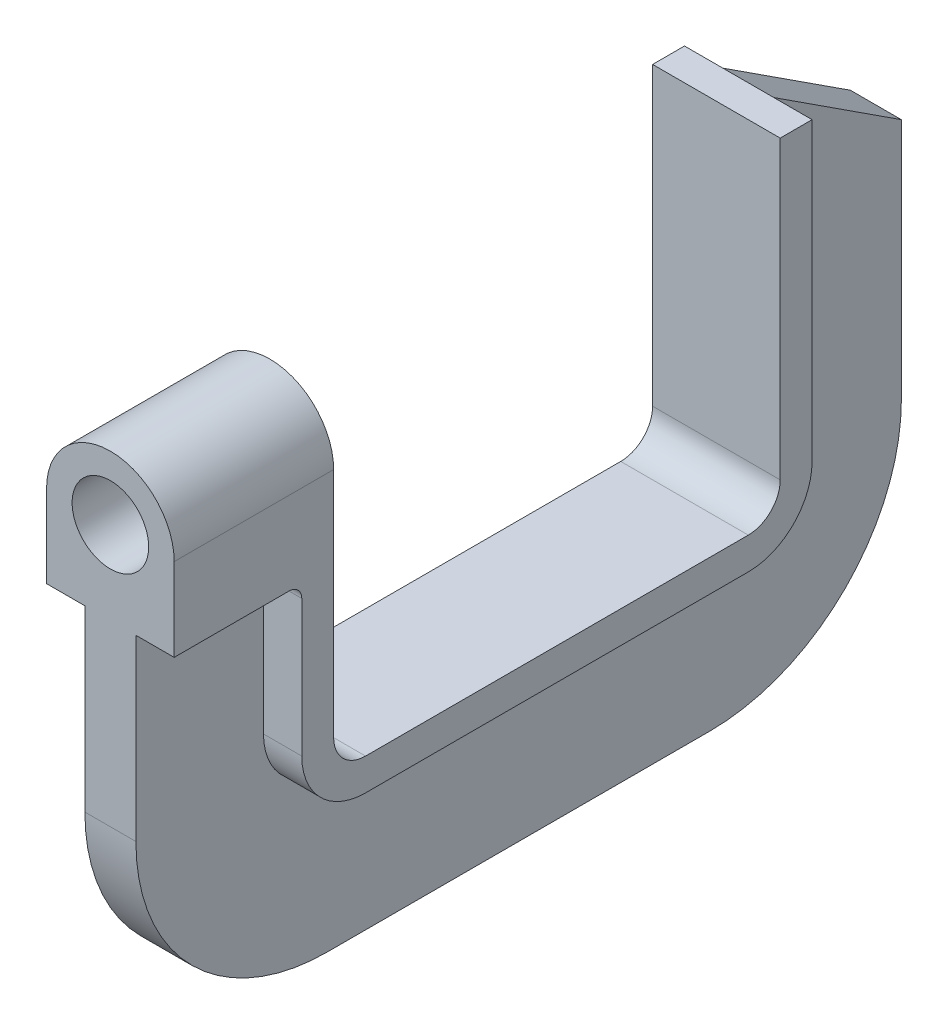
ISO-10303-21;
HEADER;
FILE_DESCRIPTION(('STEP AP214'),'2;1');
FILE_NAME('part.step','',(''),(''),'','','');
FILE_SCHEMA(('AUTOMOTIVE_DESIGN { 1 0 10303 214 1 1 1 1 }'));
ENDSEC;
DATA;
#1=APPLICATION_CONTEXT('core data for automotive mechanical design processes');
#2=APPLICATION_PROTOCOL_DEFINITION('international standard','automotive_design',2000,#1);
#3=PRODUCT_CONTEXT('',#1,'mechanical');
#4=PRODUCT('Part','Part','',(#3));
#5=PRODUCT_RELATED_PRODUCT_CATEGORY('part','',(#4));
#6=PRODUCT_DEFINITION_FORMATION('','',#4);
#7=PRODUCT_DEFINITION_CONTEXT('part definition',#1,'design');
#8=PRODUCT_DEFINITION('design','',#6,#7);
#9=PRODUCT_DEFINITION_SHAPE('','',#8);
#10=(LENGTH_UNIT() NAMED_UNIT(*) SI_UNIT(.MILLI.,.METRE.));
#11=(NAMED_UNIT(*) PLANE_ANGLE_UNIT() SI_UNIT($,.RADIAN.));
#12=(NAMED_UNIT(*) SI_UNIT($,.STERADIAN.) SOLID_ANGLE_UNIT());
#13=UNCERTAINTY_MEASURE_WITH_UNIT(LENGTH_MEASURE(1.E-05),#10,'distance_accuracy_value','');
#14=(GEOMETRIC_REPRESENTATION_CONTEXT(3) GLOBAL_UNCERTAINTY_ASSIGNED_CONTEXT((#13)) GLOBAL_UNIT_ASSIGNED_CONTEXT((#10,
#11,#12)) REPRESENTATION_CONTEXT('',''));
#15=CARTESIAN_POINT('',(0.,0.,0.));
#16=DIRECTION('',(0.,0.,1.));
#17=DIRECTION('',(1.,0.,0.));
#18=AXIS2_PLACEMENT_3D('',#15,#16,#17);
#19=CARTESIAN_POINT('',(4.,0.,70.));
#20=DIRECTION('',(0.,0.,1.));
#21=DIRECTION('',(1.,0.,0.));
#22=AXIS2_PLACEMENT_3D('',#19,#20,#21);
#23=PLANE('',#22);
#24=CARTESIAN_POINT('',(0.,-10.,70.));
#25=DIRECTION('',(0.,0.,1.));
#26=DIRECTION('',(1.,0.,0.));
#27=AXIS2_PLACEMENT_3D('',#24,#25,#26);
#28=CIRCLE('',#27,5.99999999999999);
#29=CARTESIAN_POINT('',(5.99999999999999,-10.,70.));
#30=VERTEX_POINT('',#29);
#31=EDGE_CURVE('E269',#30,#30,#28,.T.);
#32=ORIENTED_EDGE('',*,*,#31,.T.);
#33=EDGE_LOOP('',(#32));
#34=FACE_BOUND('',#33,.T.);
#35=CARTESIAN_POINT('',(0.,-10.,70.));
#36=DIRECTION('',(0.,0.,1.));
#37=DIRECTION('',(1.,0.,0.));
#38=AXIS2_PLACEMENT_3D('',#35,#36,#37);
#39=CIRCLE('',#38,10.);
#40=CARTESIAN_POINT('',(-10.,-10.,70.));
#41=VERTEX_POINT('',#40);
#42=CARTESIAN_POINT('',(10.,-10.,70.));
#43=VERTEX_POINT('',#42);
#44=EDGE_CURVE('E253',#41,#43,#39,.F.);
#45=ORIENTED_EDGE('',*,*,#44,.T.);
#46=DIRECTION('',(0.,1.,0.));
#47=VECTOR('',#46,1.);
#48=CARTESIAN_POINT('',(10.,0.,70.));
#49=LINE('',#48,#47);
#50=CARTESIAN_POINT('',(10.,-46.399278983438,70.));
#51=VERTEX_POINT('',#50);
#52=EDGE_CURVE('E268',#51,#43,#49,.T.);
#53=ORIENTED_EDGE('',*,*,#52,.F.);
#54=DIRECTION('',(-1.,0.,0.));
#55=VECTOR('',#54,1.);
#56=CARTESIAN_POINT('',(4.,-46.399278983438,70.));
#57=LINE('',#56,#55);
#58=CARTESIAN_POINT('',(-10.,-46.399278983438,70.));
#59=VERTEX_POINT('',#58);
#60=EDGE_CURVE('E351',#51,#59,#57,.T.);
#61=ORIENTED_EDGE('',*,*,#60,.T.);
#62=DIRECTION('',(0.,1.,0.));
#63=VECTOR('',#62,1.);
#64=CARTESIAN_POINT('',(-10.,0.,70.));
#65=LINE('',#64,#63);
#66=EDGE_CURVE('E266',#59,#41,#65,.T.);
#67=ORIENTED_EDGE('',*,*,#66,.T.);
#68=EDGE_LOOP('',(#45,#53,#61,#67));
#69=FACE_BOUND('',#68,.T.);
#70=ADVANCED_FACE('F70',(#34,#69),#23,.F.);
#71=CARTESIAN_POINT('',(4.,0.,95.));
#72=DIRECTION('',(0.,0.,1.));
#73=DIRECTION('',(1.,0.,0.));
#74=AXIS2_PLACEMENT_3D('',#71,#72,#73);
#75=PLANE('',#74);
#76=CARTESIAN_POINT('',(0.,-10.,95.));
#77=DIRECTION('',(0.,0.,1.));
#78=DIRECTION('',(1.,0.,0.));
#79=AXIS2_PLACEMENT_3D('',#76,#77,#78);
#80=CIRCLE('',#79,6.);
#81=CARTESIAN_POINT('',(6.,-10.,95.));
#82=VERTEX_POINT('',#81);
#83=EDGE_CURVE('E894',#82,#82,#80,.T.);
#84=ORIENTED_EDGE('',*,*,#83,.F.);
#85=EDGE_LOOP('',(#84));
#86=FACE_BOUND('',#85,.T.);
#87=DIRECTION('',(0.,1.,0.));
#88=VECTOR('',#87,1.);
#89=CARTESIAN_POINT('',(10.,-23.,95.));
#90=LINE('',#89,#88);
#91=CARTESIAN_POINT('',(10.,-23.,95.));
#92=VERTEX_POINT('',#91);
#93=CARTESIAN_POINT('',(10.,-10.,95.));
#94=VERTEX_POINT('',#93);
#95=EDGE_CURVE('E517',#92,#94,#90,.T.);
#96=ORIENTED_EDGE('',*,*,#95,.T.);
#97=CARTESIAN_POINT('',(0.,-10.,95.));
#98=DIRECTION('',(0.,0.,1.));
#99=DIRECTION('',(1.,0.,0.));
#100=AXIS2_PLACEMENT_3D('',#97,#98,#99);
#101=CIRCLE('',#100,10.);
#102=CARTESIAN_POINT('',(-10.,-10.,95.));
#103=VERTEX_POINT('',#102);
#104=EDGE_CURVE('E260',#94,#103,#101,.T.);
#105=ORIENTED_EDGE('',*,*,#104,.T.);
#106=DIRECTION('',(0.,-1.,0.));
#107=VECTOR('',#106,1.);
#108=CARTESIAN_POINT('',(-10.,-10.,95.));
#109=LINE('',#108,#107);
#110=CARTESIAN_POINT('',(-10.,-23.,95.));
#111=VERTEX_POINT('',#110);
#112=EDGE_CURVE('E513',#103,#111,#109,.T.);
#113=ORIENTED_EDGE('',*,*,#112,.T.);
#114=DIRECTION('',(1.,0.,0.));
#115=VECTOR('',#114,1.);
#116=CARTESIAN_POINT('',(-10.,-23.,95.));
#117=LINE('',#116,#115);
#118=CARTESIAN_POINT('',(-4.,-23.,95.));
#119=VERTEX_POINT('',#118);
#120=EDGE_CURVE('E448',#111,#119,#117,.T.);
#121=ORIENTED_EDGE('',*,*,#120,.T.);
#122=DIRECTION('',(0.,1.,0.));
#123=VECTOR('',#122,1.);
#124=CARTESIAN_POINT('',(-4.,0.,95.));
#125=LINE('',#124,#123);
#126=CARTESIAN_POINT('',(-4.,-50.9999999999998,95.));
#127=VERTEX_POINT('',#126);
#128=EDGE_CURVE('E368',#127,#119,#125,.T.);
#129=ORIENTED_EDGE('',*,*,#128,.F.);
#130=DIRECTION('',(-1.,0.,0.));
#131=VECTOR('',#130,1.);
#132=CARTESIAN_POINT('',(4.,-50.9999999999998,95.));
#133=LINE('',#132,#131);
#134=CARTESIAN_POINT('',(4.,-50.9999999999998,95.));
#135=VERTEX_POINT('',#134);
#136=EDGE_CURVE('E384',#135,#127,#133,.T.);
#137=ORIENTED_EDGE('',*,*,#136,.F.);
#138=DIRECTION('',(0.,1.,0.));
#139=VECTOR('',#138,1.);
#140=CARTESIAN_POINT('',(4.,0.,95.));
#141=LINE('',#140,#139);
#142=CARTESIAN_POINT('',(4.,-23.,95.));
#143=VERTEX_POINT('',#142);
#144=EDGE_CURVE('E379',#135,#143,#141,.T.);
#145=ORIENTED_EDGE('',*,*,#144,.T.);
#146=EDGE_CURVE('E552',#143,#92,#117,.T.);
#147=ORIENTED_EDGE('',*,*,#146,.T.);
#148=EDGE_LOOP('',(#96,#105,#113,#121,#129,#137,#145,#147));
#149=FACE_BOUND('',#148,.T.);
#150=ADVANCED_FACE('F553',(#86,#149),#75,.T.);
#151=CARTESIAN_POINT('',(-10.,0.,0.));
#152=DIRECTION('',(1.,0.,0.));
#153=DIRECTION('',(0.,0.,-1.));
#154=AXIS2_PLACEMENT_3D('',#151,#152,#153);
#155=PLANE('',#154);
#156=DIRECTION('',(0.,0.,1.));
#157=VECTOR('',#156,1.);
#158=CARTESIAN_POINT('',(-10.,-10.,39.5204986917437));
#159=LINE('',#158,#157);
#160=EDGE_CURVE('E455',#41,#103,#159,.T.);
#161=ORIENTED_EDGE('',*,*,#160,.F.);
#162=ORIENTED_EDGE('',*,*,#66,.F.);
#163=CARTESIAN_POINT('',(-10.,-46.399278983438,65.));
#164=DIRECTION('',(1.,0.,0.));
#165=DIRECTION('',(0.,0.,-1.));
#166=AXIS2_PLACEMENT_3D('',#163,#164,#165);
#167=CIRCLE('',#166,5.);
#168=CARTESIAN_POINT('',(-10.,-51.399278983438,65.));
#169=VERTEX_POINT('',#168);
#170=EDGE_CURVE('E307',#169,#59,#167,.F.);
#171=ORIENTED_EDGE('',*,*,#170,.F.);
#172=DIRECTION('',(0.,0.,1.));
#173=VECTOR('',#172,1.);
#174=CARTESIAN_POINT('',(-10.,-51.399278983438,0.));
#175=LINE('',#174,#173);
#176=CARTESIAN_POINT('',(-10.,-51.399278983438,5.00000000000003));
#177=VERTEX_POINT('',#176);
#178=EDGE_CURVE('E306',#177,#169,#175,.T.);
#179=ORIENTED_EDGE('',*,*,#178,.F.);
#180=CARTESIAN_POINT('',(-10.,-46.399278983438,4.99999999999999));
#181=DIRECTION('',(1.,0.,0.));
#182=DIRECTION('',(0.,0.,-1.));
#183=AXIS2_PLACEMENT_3D('',#180,#181,#182);
#184=CIRCLE('',#183,5.);
#185=CARTESIAN_POINT('',(-10.,-46.399278983438,0.));
#186=VERTEX_POINT('',#185);
#187=EDGE_CURVE('E303',#186,#177,#184,.F.);
#188=ORIENTED_EDGE('',*,*,#187,.F.);
#189=DIRECTION('',(0.,-1.,0.));
#190=VECTOR('',#189,1.);
#191=CARTESIAN_POINT('',(-10.,0.,0.));
#192=LINE('',#191,#190);
#193=CARTESIAN_POINT('',(-10.,0.,0.));
#194=VERTEX_POINT('',#193);
#195=EDGE_CURVE('E297',#194,#186,#192,.T.);
#196=ORIENTED_EDGE('',*,*,#195,.F.);
#197=DIRECTION('',(0.,0.,-1.));
#198=VECTOR('',#197,1.);
#199=CARTESIAN_POINT('',(-10.,0.,0.));
#200=LINE('',#199,#198);
#201=CARTESIAN_POINT('',(-10.,0.,-5.));
#202=VERTEX_POINT('',#201);
#203=EDGE_CURVE('E300',#194,#202,#200,.T.);
#204=ORIENTED_EDGE('',*,*,#203,.T.);
#205=DIRECTION('',(0.,-1.,0.));
#206=VECTOR('',#205,1.);
#207=CARTESIAN_POINT('',(-10.,0.,-5.));
#208=LINE('',#207,#206);
#209=CARTESIAN_POINT('',(-10.,-46.399278983438,-5.));
#210=VERTEX_POINT('',#209);
#211=EDGE_CURVE('E295',#202,#210,#208,.T.);
#212=ORIENTED_EDGE('',*,*,#211,.T.);
#213=CARTESIAN_POINT('',(-10.,-46.399278983438,4.99999999999999));
#214=DIRECTION('',(1.,0.,0.));
#215=DIRECTION('',(0.,0.,-1.));
#216=AXIS2_PLACEMENT_3D('',#213,#214,#215);
#217=CIRCLE('',#216,10.);
#218=CARTESIAN_POINT('',(-10.,-56.399278983438,5.00000000000007));
#219=VERTEX_POINT('',#218);
#220=EDGE_CURVE('E293',#210,#219,#217,.F.);
#221=ORIENTED_EDGE('',*,*,#220,.T.);
#222=DIRECTION('',(0.,0.,1.));
#223=VECTOR('',#222,1.);
#224=CARTESIAN_POINT('',(-10.,-56.399278983438,0.));
#225=LINE('',#224,#223);
#226=CARTESIAN_POINT('',(-10.,-56.399278983438,65.));
#227=VERTEX_POINT('',#226);
#228=EDGE_CURVE('E290',#219,#227,#225,.T.);
#229=ORIENTED_EDGE('',*,*,#228,.T.);
#230=CARTESIAN_POINT('',(-10.,-46.399278983438,65.));
#231=DIRECTION('',(1.,0.,0.));
#232=DIRECTION('',(0.,0.,-1.));
#233=AXIS2_PLACEMENT_3D('',#230,#231,#232);
#234=CIRCLE('',#233,9.99999999999999);
#235=CARTESIAN_POINT('',(-10.,-46.399278983438,75.));
#236=VERTEX_POINT('',#235);
#237=EDGE_CURVE('E283',#227,#236,#234,.F.);
#238=ORIENTED_EDGE('',*,*,#237,.T.);
#239=DIRECTION('',(0.,1.,0.));
#240=VECTOR('',#239,1.);
#241=CARTESIAN_POINT('',(-10.,0.,75.));
#242=LINE('',#241,#240);
#243=CARTESIAN_POINT('',(-10.,-25.,75.));
#244=VERTEX_POINT('',#243);
#245=EDGE_CURVE('E312',#236,#244,#242,.T.);
#246=ORIENTED_EDGE('',*,*,#245,.T.);
#247=CARTESIAN_POINT('',(-10.,-25.,77.));
#248=DIRECTION('',(1.,0.,0.));
#249=DIRECTION('',(0.,0.,-1.));
#250=AXIS2_PLACEMENT_3D('',#247,#248,#249);
#251=CIRCLE('',#250,2.);
#252=CARTESIAN_POINT('',(-10.,-23.,77.));
#253=VERTEX_POINT('',#252);
#254=EDGE_CURVE('E72',#244,#253,#251,.T.);
#255=ORIENTED_EDGE('',*,*,#254,.T.);
#256=DIRECTION('',(0.,0.,1.));
#257=VECTOR('',#256,1.);
#258=CARTESIAN_POINT('',(-10.,-23.,39.5204986917437));
#259=LINE('',#258,#257);
#260=EDGE_CURVE('E439',#253,#111,#259,.T.);
#261=ORIENTED_EDGE('',*,*,#260,.T.);
#262=ORIENTED_EDGE('',*,*,#112,.F.);
#263=EDGE_LOOP('',(#161,#162,#171,#179,#188,#196,#204,#212,#221,#229,#238,#246,#255,#261,#262));
#264=FACE_BOUND('',#263,.T.);
#265=ADVANCED_FACE('F438',(#264),#155,.F.);
#266=CARTESIAN_POINT('',(4.,-51.,65.));
#267=DIRECTION('',(-1.,0.,0.));
#268=DIRECTION('',(0.,0.,1.));
#269=AXIS2_PLACEMENT_3D('',#266,#267,#268);
#270=CYLINDRICAL_SURFACE('',#269,30.);
#271=CARTESIAN_POINT('',(-4.,-51.,65.));
#272=DIRECTION('',(1.,0.,0.));
#273=DIRECTION('',(0.,0.,-1.));
#274=AXIS2_PLACEMENT_3D('',#271,#272,#273);
#275=CIRCLE('',#274,30.);
#276=CARTESIAN_POINT('',(-4.,-81.,64.9999999999998));
#277=VERTEX_POINT('',#276);
#278=EDGE_CURVE('E361',#277,#127,#275,.F.);
#279=ORIENTED_EDGE('',*,*,#278,.F.);
#280=DIRECTION('',(-1.,0.,0.));
#281=VECTOR('',#280,1.);
#282=CARTESIAN_POINT('',(4.,-81.,64.9999999999998));
#283=LINE('',#282,#281);
#284=CARTESIAN_POINT('',(4.,-81.,64.9999999999998));
#285=VERTEX_POINT('',#284);
#286=EDGE_CURVE('E408',#285,#277,#283,.T.);
#287=ORIENTED_EDGE('',*,*,#286,.F.);
#288=CARTESIAN_POINT('',(4.,-51.,65.));
#289=DIRECTION('',(1.,0.,0.));
#290=DIRECTION('',(0.,0.,-1.));
#291=AXIS2_PLACEMENT_3D('',#288,#289,#290);
#292=CIRCLE('',#291,30.);
#293=EDGE_CURVE('E364',#285,#135,#292,.F.);
#294=ORIENTED_EDGE('',*,*,#293,.T.);
#295=ORIENTED_EDGE('',*,*,#136,.T.);
#296=EDGE_LOOP('',(#279,#287,#294,#295));
#297=FACE_BOUND('',#296,.T.);
#298=ADVANCED_FACE('F546',(#297),#270,.T.);
#299=CARTESIAN_POINT('',(4.,-81.,0.));
#300=DIRECTION('',(0.,-1.,0.));
#301=DIRECTION('',(0.,0.,-1.));
#302=AXIS2_PLACEMENT_3D('',#299,#300,#301);
#303=PLANE('',#302);
#304=DIRECTION('',(0.,0.,1.));
#305=VECTOR('',#304,1.);
#306=CARTESIAN_POINT('',(-4.,-81.,0.));
#307=LINE('',#306,#305);
#308=CARTESIAN_POINT('',(-4.,-81.,5.0000000000002));
#309=VERTEX_POINT('',#308);
#310=EDGE_CURVE('E387',#309,#277,#307,.T.);
#311=ORIENTED_EDGE('',*,*,#310,.F.);
#312=DIRECTION('',(-1.,0.,0.));
#313=VECTOR('',#312,1.);
#314=CARTESIAN_POINT('',(4.,-81.,5.0000000000002));
#315=LINE('',#314,#313);
#316=CARTESIAN_POINT('',(4.,-81.,5.0000000000002));
#317=VERTEX_POINT('',#316);
#318=EDGE_CURVE('E409',#317,#309,#315,.T.);
#319=ORIENTED_EDGE('',*,*,#318,.F.);
#320=DIRECTION('',(0.,0.,1.));
#321=VECTOR('',#320,1.);
#322=CARTESIAN_POINT('',(4.,-81.,0.));
#323=LINE('',#322,#321);
#324=EDGE_CURVE('E370',#317,#285,#323,.T.);
#325=ORIENTED_EDGE('',*,*,#324,.T.);
#326=ORIENTED_EDGE('',*,*,#286,.T.);
#327=EDGE_LOOP('',(#311,#319,#325,#326));
#328=FACE_BOUND('',#327,.T.);
#329=ADVANCED_FACE('F543',(#328),#303,.T.);
#330=CARTESIAN_POINT('',(4.,-51.,4.99999999999999));
#331=DIRECTION('',(-1.,0.,0.));
#332=DIRECTION('',(0.,0.,1.));
#333=AXIS2_PLACEMENT_3D('',#330,#331,#332);
#334=CYLINDRICAL_SURFACE('',#333,30.);
#335=CARTESIAN_POINT('',(-4.,-51.,4.99999999999999));
#336=DIRECTION('',(1.,0.,0.));
#337=DIRECTION('',(0.,0.,-1.));
#338=AXIS2_PLACEMENT_3D('',#335,#336,#337);
#339=CIRCLE('',#338,30.);
#340=CARTESIAN_POINT('',(-4.,-50.9999999999998,-25.));
#341=VERTEX_POINT('',#340);
#342=EDGE_CURVE('E386',#341,#309,#339,.F.);
#343=ORIENTED_EDGE('',*,*,#342,.F.);
#344=DIRECTION('',(-1.,0.,0.));
#345=VECTOR('',#344,1.);
#346=CARTESIAN_POINT('',(4.,-50.9999999999998,-25.));
#347=LINE('',#346,#345);
#348=CARTESIAN_POINT('',(4.,-50.9999999999998,-25.));
#349=VERTEX_POINT('',#348);
#350=EDGE_CURVE('E407',#349,#341,#347,.T.);
#351=ORIENTED_EDGE('',*,*,#350,.F.);
#352=CARTESIAN_POINT('',(4.,-51.,4.99999999999999));
#353=DIRECTION('',(1.,0.,0.));
#354=DIRECTION('',(0.,0.,-1.));
#355=AXIS2_PLACEMENT_3D('',#352,#353,#354);
#356=CIRCLE('',#355,30.);
#357=EDGE_CURVE('E371',#349,#317,#356,.F.);
#358=ORIENTED_EDGE('',*,*,#357,.T.);
#359=ORIENTED_EDGE('',*,*,#318,.T.);
#360=EDGE_LOOP('',(#343,#351,#358,#359));
#361=FACE_BOUND('',#360,.T.);
#362=ADVANCED_FACE('F545',(#361),#334,.T.);
#363=CARTESIAN_POINT('',(4.,0.,-25.));
#364=DIRECTION('',(0.,0.,-1.));
#365=DIRECTION('',(-1.,0.,0.));
#366=AXIS2_PLACEMENT_3D('',#363,#364,#365);
#367=PLANE('',#366);
#368=DIRECTION('',(0.,-1.,0.));
#369=VECTOR('',#368,1.);
#370=CARTESIAN_POINT('',(-4.,0.,-25.));
#371=LINE('',#370,#369);
#372=CARTESIAN_POINT('',(-4.,-13.,-25.));
#373=VERTEX_POINT('',#372);
#374=EDGE_CURVE('E395',#373,#341,#371,.T.);
#375=ORIENTED_EDGE('',*,*,#374,.F.);
#376=DIRECTION('',(-1.,0.,0.));
#377=VECTOR('',#376,1.);
#378=CARTESIAN_POINT('',(4.,-13.,-25.));
#379=LINE('',#378,#377);
#380=CARTESIAN_POINT('',(4.,-13.,-25.));
#381=VERTEX_POINT('',#380);
#382=EDGE_CURVE('E404',#381,#373,#379,.T.);
#383=ORIENTED_EDGE('',*,*,#382,.F.);
#384=DIRECTION('',(0.,-1.,0.));
#385=VECTOR('',#384,1.);
#386=CARTESIAN_POINT('',(4.,0.,-25.));
#387=LINE('',#386,#385);
#388=EDGE_CURVE('E372',#381,#349,#387,.T.);
#389=ORIENTED_EDGE('',*,*,#388,.T.);
#390=ORIENTED_EDGE('',*,*,#350,.T.);
#391=EDGE_LOOP('',(#375,#383,#389,#390));
#392=FACE_BOUND('',#391,.T.);
#393=ADVANCED_FACE('F539',(#392),#367,.T.);
#394=CARTESIAN_POINT('',(4.,2.28471001757469,-1.48506151142355));
#395=DIRECTION('',(0.,0.838443616300637,-0.544988350595414));
#396=DIRECTION('',(0.,0.544988350595414,0.838443616300637));
#397=AXIS2_PLACEMENT_3D('',#394,#395,#396);
#398=PLANE('',#397);
#399=DIRECTION('',(0.,-0.544988350595414,-0.838443616300637));
#400=VECTOR('',#399,1.);
#401=CARTESIAN_POINT('',(-4.,2.28471001757469,-1.48506151142355));
#402=LINE('',#401,#400);
#403=CARTESIAN_POINT('',(-4.,0.,-5.));
#404=VERTEX_POINT('',#403);
#405=EDGE_CURVE('E394',#404,#373,#402,.T.);
#406=ORIENTED_EDGE('',*,*,#405,.F.);
#407=DIRECTION('',(-1.,0.,0.));
#408=VECTOR('',#407,1.);
#409=CARTESIAN_POINT('',(4.,0.,-5.));
#410=LINE('',#409,#408);
#411=CARTESIAN_POINT('',(4.,0.,-5.));
#412=VERTEX_POINT('',#411);
#413=EDGE_CURVE('E402',#412,#404,#410,.T.);
#414=ORIENTED_EDGE('',*,*,#413,.F.);
#415=DIRECTION('',(0.,-0.544988350595414,-0.838443616300637));
#416=VECTOR('',#415,1.);
#417=CARTESIAN_POINT('',(4.,2.28471001757469,-1.48506151142355));
#418=LINE('',#417,#416);
#419=EDGE_CURVE('E380',#412,#381,#418,.T.);
#420=ORIENTED_EDGE('',*,*,#419,.T.);
#421=ORIENTED_EDGE('',*,*,#382,.T.);
#422=EDGE_LOOP('',(#406,#414,#420,#421));
#423=FACE_BOUND('',#422,.T.);
#424=ADVANCED_FACE('F478',(#423),#398,.T.);
#425=CARTESIAN_POINT('',(4.,0.,0.));
#426=DIRECTION('',(1.,0.,0.));
#427=DIRECTION('',(0.,0.,-1.));
#428=AXIS2_PLACEMENT_3D('',#425,#426,#427);
#429=PLANE('',#428);
#430=DIRECTION('',(0.,-1.,0.));
#431=VECTOR('',#430,1.);
#432=CARTESIAN_POINT('',(4.,0.,75.));
#433=LINE('',#432,#431);
#434=CARTESIAN_POINT('',(4.,-25.,75.));
#435=VERTEX_POINT('',#434);
#436=CARTESIAN_POINT('',(4.,-46.399278983438,75.));
#437=VERTEX_POINT('',#436);
#438=EDGE_CURVE('E345',#435,#437,#433,.T.);
#439=ORIENTED_EDGE('',*,*,#438,.F.);
#440=CARTESIAN_POINT('',(4.,-25.,77.));
#441=DIRECTION('',(1.,0.,0.));
#442=DIRECTION('',(0.,0.,-1.));
#443=AXIS2_PLACEMENT_3D('',#440,#441,#442);
#444=CIRCLE('',#443,2.);
#445=CARTESIAN_POINT('',(4.,-23.,77.));
#446=VERTEX_POINT('',#445);
#447=EDGE_CURVE('E432',#435,#446,#444,.T.);
#448=ORIENTED_EDGE('',*,*,#447,.T.);
#449=DIRECTION('',(0.,0.,-1.));
#450=VECTOR('',#449,1.);
#451=CARTESIAN_POINT('',(4.,-23.,0.));
#452=LINE('',#451,#450);
#453=EDGE_CURVE('E261',#143,#446,#452,.T.);
#454=ORIENTED_EDGE('',*,*,#453,.F.);
#455=ORIENTED_EDGE('',*,*,#144,.F.);
#456=ORIENTED_EDGE('',*,*,#293,.F.);
#457=ORIENTED_EDGE('',*,*,#324,.F.);
#458=ORIENTED_EDGE('',*,*,#357,.F.);
#459=ORIENTED_EDGE('',*,*,#388,.F.);
#460=ORIENTED_EDGE('',*,*,#419,.F.);
#461=DIRECTION('',(0.,1.,0.));
#462=VECTOR('',#461,1.);
#463=CARTESIAN_POINT('',(4.,0.,-5.));
#464=LINE('',#463,#462);
#465=CARTESIAN_POINT('',(4.,-46.399278983438,-5.));
#466=VERTEX_POINT('',#465);
#467=EDGE_CURVE('E339',#466,#412,#464,.T.);
#468=ORIENTED_EDGE('',*,*,#467,.F.);
#469=CARTESIAN_POINT('',(4.,-46.399278983438,4.99999999999999));
#470=DIRECTION('',(1.,0.,0.));
#471=DIRECTION('',(0.,0.,-1.));
#472=AXIS2_PLACEMENT_3D('',#469,#470,#471);
#473=CIRCLE('',#472,10.);
#474=CARTESIAN_POINT('',(4.,-56.399278983438,5.00000000000007));
#475=VERTEX_POINT('',#474);
#476=EDGE_CURVE('E341',#475,#466,#473,.T.);
#477=ORIENTED_EDGE('',*,*,#476,.F.);
#478=DIRECTION('',(0.,0.,-1.));
#479=VECTOR('',#478,1.);
#480=CARTESIAN_POINT('',(4.,-56.399278983438,0.));
#481=LINE('',#480,#479);
#482=CARTESIAN_POINT('',(4.,-56.399278983438,65.));
#483=VERTEX_POINT('',#482);
#484=EDGE_CURVE('E350',#483,#475,#481,.T.);
#485=ORIENTED_EDGE('',*,*,#484,.F.);
#486=CARTESIAN_POINT('',(4.,-46.399278983438,65.));
#487=DIRECTION('',(1.,0.,0.));
#488=DIRECTION('',(0.,0.,-1.));
#489=AXIS2_PLACEMENT_3D('',#486,#487,#488);
#490=CIRCLE('',#489,9.99999999999999);
#491=EDGE_CURVE('E349',#437,#483,#490,.T.);
#492=ORIENTED_EDGE('',*,*,#491,.F.);
#493=EDGE_LOOP('',(#439,#448,#454,#455,#456,#457,#458,#459,#460,#468,#477,#485,#492));
#494=FACE_BOUND('',#493,.T.);
#495=ADVANCED_FACE('F535',(#494),#429,.T.);
#496=CARTESIAN_POINT('',(-4.,0.,0.));
#497=DIRECTION('',(1.,0.,0.));
#498=DIRECTION('',(0.,0.,-1.));
#499=AXIS2_PLACEMENT_3D('',#496,#497,#498);
#500=PLANE('',#499);
#501=DIRECTION('',(0.,0.,-1.));
#502=VECTOR('',#501,1.);
#503=CARTESIAN_POINT('',(-4.,-23.,0.));
#504=LINE('',#503,#502);
#505=CARTESIAN_POINT('',(-4.,-23.,77.));
#506=VERTEX_POINT('',#505);
#507=EDGE_CURVE('E286',#119,#506,#504,.T.);
#508=ORIENTED_EDGE('',*,*,#507,.T.);
#509=CARTESIAN_POINT('',(-4.,-25.,77.));
#510=DIRECTION('',(1.,0.,0.));
#511=DIRECTION('',(0.,0.,-1.));
#512=AXIS2_PLACEMENT_3D('',#509,#510,#511);
#513=CIRCLE('',#512,2.);
#514=CARTESIAN_POINT('',(-4.,-25.,75.));
#515=VERTEX_POINT('',#514);
#516=EDGE_CURVE('E428',#506,#515,#513,.F.);
#517=ORIENTED_EDGE('',*,*,#516,.T.);
#518=DIRECTION('',(0.,-1.,0.));
#519=VECTOR('',#518,1.);
#520=CARTESIAN_POINT('',(-4.,0.,75.));
#521=LINE('',#520,#519);
#522=CARTESIAN_POINT('',(-4.,-46.399278983438,75.));
#523=VERTEX_POINT('',#522);
#524=EDGE_CURVE('E415',#515,#523,#521,.T.);
#525=ORIENTED_EDGE('',*,*,#524,.T.);
#526=CARTESIAN_POINT('',(-4.,-46.399278983438,65.));
#527=DIRECTION('',(1.,0.,0.));
#528=DIRECTION('',(0.,0.,-1.));
#529=AXIS2_PLACEMENT_3D('',#526,#527,#528);
#530=CIRCLE('',#529,9.99999999999999);
#531=CARTESIAN_POINT('',(-4.,-56.399278983438,65.));
#532=VERTEX_POINT('',#531);
#533=EDGE_CURVE('E413',#523,#532,#530,.T.);
#534=ORIENTED_EDGE('',*,*,#533,.T.);
#535=DIRECTION('',(0.,0.,-1.));
#536=VECTOR('',#535,1.);
#537=CARTESIAN_POINT('',(-4.,-56.399278983438,0.));
#538=LINE('',#537,#536);
#539=CARTESIAN_POINT('',(-4.,-56.399278983438,5.00000000000007));
#540=VERTEX_POINT('',#539);
#541=EDGE_CURVE('E420',#532,#540,#538,.T.);
#542=ORIENTED_EDGE('',*,*,#541,.T.);
#543=CARTESIAN_POINT('',(-4.,-46.399278983438,4.99999999999999));
#544=DIRECTION('',(1.,0.,0.));
#545=DIRECTION('',(0.,0.,-1.));
#546=AXIS2_PLACEMENT_3D('',#543,#544,#545);
#547=CIRCLE('',#546,10.);
#548=CARTESIAN_POINT('',(-4.,-46.399278983438,-5.));
#549=VERTEX_POINT('',#548);
#550=EDGE_CURVE('E417',#540,#549,#547,.T.);
#551=ORIENTED_EDGE('',*,*,#550,.T.);
#552=DIRECTION('',(0.,1.,0.));
#553=VECTOR('',#552,1.);
#554=CARTESIAN_POINT('',(-4.,0.,-5.));
#555=LINE('',#554,#553);
#556=EDGE_CURVE('E337',#549,#404,#555,.T.);
#557=ORIENTED_EDGE('',*,*,#556,.T.);
#558=ORIENTED_EDGE('',*,*,#405,.T.);
#559=ORIENTED_EDGE('',*,*,#374,.T.);
#560=ORIENTED_EDGE('',*,*,#342,.T.);
#561=ORIENTED_EDGE('',*,*,#310,.T.);
#562=ORIENTED_EDGE('',*,*,#278,.T.);
#563=ORIENTED_EDGE('',*,*,#128,.T.);
#564=EDGE_LOOP('',(#508,#517,#525,#534,#542,#551,#557,#558,#559,#560,#561,#562,#563));
#565=FACE_BOUND('',#564,.T.);
#566=ADVANCED_FACE('F460',(#565),#500,.F.);
#567=CARTESIAN_POINT('',(4.,0.,0.));
#568=DIRECTION('',(0.,1.,0.));
#569=DIRECTION('',(0.,0.,1.));
#570=AXIS2_PLACEMENT_3D('',#567,#568,#569);
#571=PLANE('',#570);
#572=ORIENTED_EDGE('',*,*,#413,.T.);
#573=DIRECTION('',(-1.,0.,0.));
#574=VECTOR('',#573,1.);
#575=CARTESIAN_POINT('',(10.,0.,-5.));
#576=LINE('',#575,#574);
#577=EDGE_CURVE('E318',#404,#202,#576,.T.);
#578=ORIENTED_EDGE('',*,*,#577,.T.);
#579=ORIENTED_EDGE('',*,*,#203,.F.);
#580=DIRECTION('',(-1.,0.,0.));
#581=VECTOR('',#580,1.);
#582=CARTESIAN_POINT('',(4.,0.,0.));
#583=LINE('',#582,#581);
#584=CARTESIAN_POINT('',(10.,0.,0.));
#585=VERTEX_POINT('',#584);
#586=EDGE_CURVE('E363',#585,#194,#583,.T.);
#587=ORIENTED_EDGE('',*,*,#586,.F.);
#588=DIRECTION('',(0.,0.,-1.));
#589=VECTOR('',#588,1.);
#590=CARTESIAN_POINT('',(10.,0.,0.));
#591=LINE('',#590,#589);
#592=CARTESIAN_POINT('',(10.,0.,-5.));
#593=VERTEX_POINT('',#592);
#594=EDGE_CURVE('E487',#585,#593,#591,.T.);
#595=ORIENTED_EDGE('',*,*,#594,.T.);
#596=EDGE_CURVE('E322',#593,#412,#576,.T.);
#597=ORIENTED_EDGE('',*,*,#596,.T.);
#598=EDGE_LOOP('',(#572,#578,#579,#587,#595,#597));
#599=FACE_BOUND('',#598,.T.);
#600=ADVANCED_FACE('F481',(#599),#571,.T.);
#601=CARTESIAN_POINT('',(4.,0.,0.));
#602=DIRECTION('',(0.,0.,-1.));
#603=DIRECTION('',(0.,1.,0.));
#604=AXIS2_PLACEMENT_3D('',#601,#602,#603);
#605=PLANE('',#604);
#606=ORIENTED_EDGE('',*,*,#586,.T.);
#607=ORIENTED_EDGE('',*,*,#195,.T.);
#608=DIRECTION('',(-1.,0.,0.));
#609=VECTOR('',#608,1.);
#610=CARTESIAN_POINT('',(4.,-46.399278983438,0.));
#611=LINE('',#610,#609);
#612=CARTESIAN_POINT('',(10.,-46.399278983438,0.));
#613=VERTEX_POINT('',#612);
#614=EDGE_CURVE('E360',#613,#186,#611,.T.);
#615=ORIENTED_EDGE('',*,*,#614,.F.);
#616=DIRECTION('',(0.,-1.,0.));
#617=VECTOR('',#616,1.);
#618=CARTESIAN_POINT('',(10.,0.,0.));
#619=LINE('',#618,#617);
#620=EDGE_CURVE('E497',#585,#613,#619,.T.);
#621=ORIENTED_EDGE('',*,*,#620,.F.);
#622=EDGE_LOOP('',(#606,#607,#615,#621));
#623=FACE_BOUND('',#622,.T.);
#624=ADVANCED_FACE('F595',(#623),#605,.F.);
#625=CARTESIAN_POINT('',(4.,-46.399278983438,4.99999999999999));
#626=DIRECTION('',(-1.,0.,0.));
#627=DIRECTION('',(0.,0.,1.));
#628=AXIS2_PLACEMENT_3D('',#625,#626,#627);
#629=CYLINDRICAL_SURFACE('',#628,5.);
#630=ORIENTED_EDGE('',*,*,#614,.T.);
#631=ORIENTED_EDGE('',*,*,#187,.T.);
#632=DIRECTION('',(-1.,0.,0.));
#633=VECTOR('',#632,1.);
#634=CARTESIAN_POINT('',(4.,-51.399278983438,5.00000000000003));
#635=LINE('',#634,#633);
#636=CARTESIAN_POINT('',(10.,-51.399278983438,5.00000000000003));
#637=VERTEX_POINT('',#636);
#638=EDGE_CURVE('E357',#637,#177,#635,.T.);
#639=ORIENTED_EDGE('',*,*,#638,.F.);
#640=CARTESIAN_POINT('',(10.,-46.399278983438,4.99999999999999));
#641=DIRECTION('',(1.,0.,0.));
#642=DIRECTION('',(0.,0.,-1.));
#643=AXIS2_PLACEMENT_3D('',#640,#641,#642);
#644=CIRCLE('',#643,5.);
#645=EDGE_CURVE('E506',#613,#637,#644,.F.);
#646=ORIENTED_EDGE('',*,*,#645,.F.);
#647=EDGE_LOOP('',(#630,#631,#639,#646));
#648=FACE_BOUND('',#647,.T.);
#649=ADVANCED_FACE('F588',(#648),#629,.F.);
#650=CARTESIAN_POINT('',(4.,-51.399278983438,0.));
#651=DIRECTION('',(0.,-1.,0.));
#652=DIRECTION('',(0.,0.,-1.));
#653=AXIS2_PLACEMENT_3D('',#650,#651,#652);
#654=PLANE('',#653);
#655=ORIENTED_EDGE('',*,*,#638,.T.);
#656=ORIENTED_EDGE('',*,*,#178,.T.);
#657=DIRECTION('',(-1.,0.,0.));
#658=VECTOR('',#657,1.);
#659=CARTESIAN_POINT('',(4.,-51.399278983438,65.));
#660=LINE('',#659,#658);
#661=CARTESIAN_POINT('',(10.,-51.399278983438,65.));
#662=VERTEX_POINT('',#661);
#663=EDGE_CURVE('E352',#662,#169,#660,.T.);
#664=ORIENTED_EDGE('',*,*,#663,.F.);
#665=DIRECTION('',(0.,0.,1.));
#666=VECTOR('',#665,1.);
#667=CARTESIAN_POINT('',(10.,-51.399278983438,0.));
#668=LINE('',#667,#666);
#669=EDGE_CURVE('E278',#637,#662,#668,.T.);
#670=ORIENTED_EDGE('',*,*,#669,.F.);
#671=EDGE_LOOP('',(#655,#656,#664,#670));
#672=FACE_BOUND('',#671,.T.);
#673=ADVANCED_FACE('F586',(#672),#654,.F.);
#674=CARTESIAN_POINT('',(4.,-46.399278983438,65.));
#675=DIRECTION('',(-1.,0.,0.));
#676=DIRECTION('',(0.,0.,1.));
#677=AXIS2_PLACEMENT_3D('',#674,#675,#676);
#678=CYLINDRICAL_SURFACE('',#677,5.);
#679=ORIENTED_EDGE('',*,*,#663,.T.);
#680=ORIENTED_EDGE('',*,*,#170,.T.);
#681=ORIENTED_EDGE('',*,*,#60,.F.);
#682=CARTESIAN_POINT('',(10.,-46.399278983438,65.));
#683=DIRECTION('',(1.,0.,0.));
#684=DIRECTION('',(0.,0.,-1.));
#685=AXIS2_PLACEMENT_3D('',#682,#683,#684);
#686=CIRCLE('',#685,5.);
#687=EDGE_CURVE('E273',#662,#51,#686,.F.);
#688=ORIENTED_EDGE('',*,*,#687,.F.);
#689=EDGE_LOOP('',(#679,#680,#681,#688));
#690=FACE_BOUND('',#689,.T.);
#691=ADVANCED_FACE('F515',(#690),#678,.F.);
#692=CARTESIAN_POINT('',(10.,0.,75.));
#693=DIRECTION('',(0.,0.,1.));
#694=DIRECTION('',(0.,-1.,0.));
#695=AXIS2_PLACEMENT_3D('',#692,#693,#694);
#696=PLANE('',#695);
#697=ORIENTED_EDGE('',*,*,#524,.F.);
#698=DIRECTION('',(1.,0.,0.));
#699=VECTOR('',#698,1.);
#700=CARTESIAN_POINT('',(-10.,-25.,75.));
#701=LINE('',#700,#699);
#702=EDGE_CURVE('E426',#515,#244,#701,.F.);
#703=ORIENTED_EDGE('',*,*,#702,.T.);
#704=ORIENTED_EDGE('',*,*,#245,.F.);
#705=DIRECTION('',(-1.,0.,0.));
#706=VECTOR('',#705,1.);
#707=CARTESIAN_POINT('',(10.,-46.399278983438,75.));
#708=LINE('',#707,#706);
#709=EDGE_CURVE('E279',#523,#236,#708,.T.);
#710=ORIENTED_EDGE('',*,*,#709,.F.);
#711=EDGE_LOOP('',(#697,#703,#704,#710));
#712=FACE_BOUND('',#711,.T.);
#713=ADVANCED_FACE('F459',(#712),#696,.T.);
#714=CARTESIAN_POINT('',(10.,0.,-5.));
#715=DIRECTION('',(0.,0.,-1.));
#716=DIRECTION('',(-1.,0.,0.));
#717=AXIS2_PLACEMENT_3D('',#714,#715,#716);
#718=PLANE('',#717);
#719=ORIENTED_EDGE('',*,*,#556,.F.);
#720=DIRECTION('',(-1.,0.,0.));
#721=VECTOR('',#720,1.);
#722=CARTESIAN_POINT('',(10.,-46.399278983438,-5.));
#723=LINE('',#722,#721);
#724=EDGE_CURVE('E321',#549,#210,#723,.T.);
#725=ORIENTED_EDGE('',*,*,#724,.T.);
#726=ORIENTED_EDGE('',*,*,#211,.F.);
#727=ORIENTED_EDGE('',*,*,#577,.F.);
#728=EDGE_LOOP('',(#719,#725,#726,#727));
#729=FACE_BOUND('',#728,.T.);
#730=ADVANCED_FACE('F476',(#729),#718,.T.);
#731=CARTESIAN_POINT('',(10.,-46.399278983438,4.99999999999999));
#732=DIRECTION('',(-1.,0.,0.));
#733=DIRECTION('',(0.,0.,1.));
#734=AXIS2_PLACEMENT_3D('',#731,#732,#733);
#735=CYLINDRICAL_SURFACE('',#734,10.);
#736=ORIENTED_EDGE('',*,*,#550,.F.);
#737=DIRECTION('',(-1.,0.,0.));
#738=VECTOR('',#737,1.);
#739=CARTESIAN_POINT('',(10.,-56.399278983438,5.00000000000007));
#740=LINE('',#739,#738);
#741=EDGE_CURVE('E327',#540,#219,#740,.T.);
#742=ORIENTED_EDGE('',*,*,#741,.T.);
#743=ORIENTED_EDGE('',*,*,#220,.F.);
#744=ORIENTED_EDGE('',*,*,#724,.F.);
#745=EDGE_LOOP('',(#736,#742,#743,#744));
#746=FACE_BOUND('',#745,.T.);
#747=ADVANCED_FACE('F475',(#746),#735,.T.);
#748=CARTESIAN_POINT('',(10.,-56.399278983438,0.));
#749=DIRECTION('',(0.,-1.,0.));
#750=DIRECTION('',(0.,0.,-1.));
#751=AXIS2_PLACEMENT_3D('',#748,#749,#750);
#752=PLANE('',#751);
#753=ORIENTED_EDGE('',*,*,#541,.F.);
#754=DIRECTION('',(-1.,0.,0.));
#755=VECTOR('',#754,1.);
#756=CARTESIAN_POINT('',(10.,-56.399278983438,65.));
#757=LINE('',#756,#755);
#758=EDGE_CURVE('E335',#532,#227,#757,.T.);
#759=ORIENTED_EDGE('',*,*,#758,.T.);
#760=ORIENTED_EDGE('',*,*,#228,.F.);
#761=ORIENTED_EDGE('',*,*,#741,.F.);
#762=EDGE_LOOP('',(#753,#759,#760,#761));
#763=FACE_BOUND('',#762,.T.);
#764=ADVANCED_FACE('F466',(#763),#752,.T.);
#765=CARTESIAN_POINT('',(10.,-46.399278983438,65.));
#766=DIRECTION('',(-1.,0.,0.));
#767=DIRECTION('',(0.,0.,1.));
#768=AXIS2_PLACEMENT_3D('',#765,#766,#767);
#769=CYLINDRICAL_SURFACE('',#768,9.99999999999999);
#770=ORIENTED_EDGE('',*,*,#533,.F.);
#771=ORIENTED_EDGE('',*,*,#709,.T.);
#772=ORIENTED_EDGE('',*,*,#237,.F.);
#773=ORIENTED_EDGE('',*,*,#758,.F.);
#774=EDGE_LOOP('',(#770,#771,#772,#773));
#775=FACE_BOUND('',#774,.T.);
#776=ADVANCED_FACE('F462',(#775),#769,.T.);
#777=CARTESIAN_POINT('',(10.,-46.399278983438,75.));
#778=VERTEX_POINT('',#777);
#779=EDGE_CURVE('E320',#778,#437,#708,.T.);
#780=ORIENTED_EDGE('',*,*,#779,.T.);
#781=ORIENTED_EDGE('',*,*,#491,.T.);
#782=CARTESIAN_POINT('',(10.,-56.399278983438,65.));
#783=VERTEX_POINT('',#782);
#784=EDGE_CURVE('E331',#783,#483,#757,.T.);
#785=ORIENTED_EDGE('',*,*,#784,.F.);
#786=CARTESIAN_POINT('',(10.,-46.399278983438,65.));
#787=DIRECTION('',(1.,0.,0.));
#788=DIRECTION('',(0.,0.,-1.));
#789=AXIS2_PLACEMENT_3D('',#786,#787,#788);
#790=CIRCLE('',#789,9.99999999999999);
#791=EDGE_CURVE('E317',#783,#778,#790,.F.);
#792=ORIENTED_EDGE('',*,*,#791,.T.);
#793=EDGE_LOOP('',(#780,#781,#785,#792));
#794=FACE_BOUND('',#793,.T.);
#795=ADVANCED_FACE('F585',(#794),#769,.T.);
#796=ORIENTED_EDGE('',*,*,#784,.T.);
#797=ORIENTED_EDGE('',*,*,#484,.T.);
#798=CARTESIAN_POINT('',(10.,-56.399278983438,5.00000000000007));
#799=VERTEX_POINT('',#798);
#800=EDGE_CURVE('E328',#799,#475,#740,.T.);
#801=ORIENTED_EDGE('',*,*,#800,.F.);
#802=DIRECTION('',(0.,0.,1.));
#803=VECTOR('',#802,1.);
#804=CARTESIAN_POINT('',(10.,-56.399278983438,0.));
#805=LINE('',#804,#803);
#806=EDGE_CURVE('E501',#799,#783,#805,.T.);
#807=ORIENTED_EDGE('',*,*,#806,.T.);
#808=EDGE_LOOP('',(#796,#797,#801,#807));
#809=FACE_BOUND('',#808,.T.);
#810=ADVANCED_FACE('F530',(#809),#752,.T.);
#811=ORIENTED_EDGE('',*,*,#800,.T.);
#812=ORIENTED_EDGE('',*,*,#476,.T.);
#813=CARTESIAN_POINT('',(10.,-46.399278983438,-5.));
#814=VERTEX_POINT('',#813);
#815=EDGE_CURVE('E323',#814,#466,#723,.T.);
#816=ORIENTED_EDGE('',*,*,#815,.F.);
#817=CARTESIAN_POINT('',(10.,-46.399278983438,4.99999999999999));
#818=DIRECTION('',(1.,0.,0.));
#819=DIRECTION('',(0.,0.,-1.));
#820=AXIS2_PLACEMENT_3D('',#817,#818,#819);
#821=CIRCLE('',#820,10.);
#822=EDGE_CURVE('E500',#814,#799,#821,.F.);
#823=ORIENTED_EDGE('',*,*,#822,.T.);
#824=EDGE_LOOP('',(#811,#812,#816,#823));
#825=FACE_BOUND('',#824,.T.);
#826=ADVANCED_FACE('F527',(#825),#735,.T.);
#827=ORIENTED_EDGE('',*,*,#815,.T.);
#828=ORIENTED_EDGE('',*,*,#467,.T.);
#829=ORIENTED_EDGE('',*,*,#596,.F.);
#830=DIRECTION('',(0.,-1.,0.));
#831=VECTOR('',#830,1.);
#832=CARTESIAN_POINT('',(10.,0.,-5.));
#833=LINE('',#832,#831);
#834=EDGE_CURVE('E495',#593,#814,#833,.T.);
#835=ORIENTED_EDGE('',*,*,#834,.T.);
#836=EDGE_LOOP('',(#827,#828,#829,#835));
#837=FACE_BOUND('',#836,.T.);
#838=ADVANCED_FACE('F493',(#837),#718,.T.);
#839=DIRECTION('',(0.,1.,0.));
#840=VECTOR('',#839,1.);
#841=CARTESIAN_POINT('',(10.,0.,75.));
#842=LINE('',#841,#840);
#843=CARTESIAN_POINT('',(10.,-25.,75.));
#844=VERTEX_POINT('',#843);
#845=EDGE_CURVE('E277',#778,#844,#842,.T.);
#846=ORIENTED_EDGE('',*,*,#845,.T.);
#847=DIRECTION('',(1.,0.,0.));
#848=VECTOR('',#847,1.);
#849=CARTESIAN_POINT('',(4.,-25.,75.));
#850=LINE('',#849,#848);
#851=EDGE_CURVE('E90',#844,#435,#850,.F.);
#852=ORIENTED_EDGE('',*,*,#851,.T.);
#853=ORIENTED_EDGE('',*,*,#438,.T.);
#854=ORIENTED_EDGE('',*,*,#779,.F.);
#855=EDGE_LOOP('',(#846,#852,#853,#854));
#856=FACE_BOUND('',#855,.T.);
#857=ADVANCED_FACE('F625',(#856),#696,.T.);
#858=CARTESIAN_POINT('',(10.,0.,0.));
#859=DIRECTION('',(1.,0.,0.));
#860=DIRECTION('',(0.,0.,-1.));
#861=AXIS2_PLACEMENT_3D('',#858,#859,#860);
#862=PLANE('',#861);
#863=ORIENTED_EDGE('',*,*,#52,.T.);
#864=DIRECTION('',(0.,0.,1.));
#865=VECTOR('',#864,1.);
#866=CARTESIAN_POINT('',(10.,-10.,39.5204986917437));
#867=LINE('',#866,#865);
#868=EDGE_CURVE('E252',#43,#94,#867,.T.);
#869=ORIENTED_EDGE('',*,*,#868,.T.);
#870=ORIENTED_EDGE('',*,*,#95,.F.);
#871=DIRECTION('',(0.,0.,1.));
#872=VECTOR('',#871,1.);
#873=CARTESIAN_POINT('',(10.,-23.,39.5204986917437));
#874=LINE('',#873,#872);
#875=CARTESIAN_POINT('',(10.,-23.,77.));
#876=VERTEX_POINT('',#875);
#877=EDGE_CURVE('E265',#876,#92,#874,.T.);
#878=ORIENTED_EDGE('',*,*,#877,.F.);
#879=CARTESIAN_POINT('',(10.,-25.,77.));
#880=DIRECTION('',(1.,0.,0.));
#881=DIRECTION('',(0.,0.,-1.));
#882=AXIS2_PLACEMENT_3D('',#879,#880,#881);
#883=CIRCLE('',#882,2.);
#884=EDGE_CURVE('E12',#876,#844,#883,.F.);
#885=ORIENTED_EDGE('',*,*,#884,.T.);
#886=ORIENTED_EDGE('',*,*,#845,.F.);
#887=ORIENTED_EDGE('',*,*,#791,.F.);
#888=ORIENTED_EDGE('',*,*,#806,.F.);
#889=ORIENTED_EDGE('',*,*,#822,.F.);
#890=ORIENTED_EDGE('',*,*,#834,.F.);
#891=ORIENTED_EDGE('',*,*,#594,.F.);
#892=ORIENTED_EDGE('',*,*,#620,.T.);
#893=ORIENTED_EDGE('',*,*,#645,.T.);
#894=ORIENTED_EDGE('',*,*,#669,.T.);
#895=ORIENTED_EDGE('',*,*,#687,.T.);
#896=EDGE_LOOP('',(#863,#869,#870,#878,#885,#886,#887,#888,#889,#890,#891,#892,#893,#894,#895));
#897=FACE_BOUND('',#896,.T.);
#898=ADVANCED_FACE('F275',(#897),#862,.T.);
#899=CARTESIAN_POINT('',(-10.,-23.,39.5204986917437));
#900=DIRECTION('',(0.,-1.,0.));
#901=DIRECTION('',(0.,0.,-1.));
#902=AXIS2_PLACEMENT_3D('',#899,#900,#901);
#903=PLANE('',#902);
#904=ORIENTED_EDGE('',*,*,#453,.T.);
#905=DIRECTION('',(1.,0.,0.));
#906=VECTOR('',#905,1.);
#907=CARTESIAN_POINT('',(10.,-23.,77.));
#908=LINE('',#907,#906);
#909=EDGE_CURVE('E427',#446,#876,#908,.T.);
#910=ORIENTED_EDGE('',*,*,#909,.T.);
#911=ORIENTED_EDGE('',*,*,#877,.T.);
#912=ORIENTED_EDGE('',*,*,#146,.F.);
#913=EDGE_LOOP('',(#904,#910,#911,#912));
#914=FACE_BOUND('',#913,.T.);
#915=ADVANCED_FACE('F559',(#914),#903,.T.);
#916=CARTESIAN_POINT('',(0.,-10.,39.5204986917437));
#917=DIRECTION('',(0.,0.,1.));
#918=DIRECTION('',(1.,0.,0.));
#919=AXIS2_PLACEMENT_3D('',#916,#917,#918);
#920=CYLINDRICAL_SURFACE('',#919,10.);
#921=ORIENTED_EDGE('',*,*,#104,.F.);
#922=ORIENTED_EDGE('',*,*,#868,.F.);
#923=ORIENTED_EDGE('',*,*,#44,.F.);
#924=ORIENTED_EDGE('',*,*,#160,.T.);
#925=EDGE_LOOP('',(#921,#922,#923,#924));
#926=FACE_BOUND('',#925,.T.);
#927=ADVANCED_FACE('F254',(#926),#920,.T.);
#928=ORIENTED_EDGE('',*,*,#260,.F.);
#929=DIRECTION('',(1.,0.,0.));
#930=VECTOR('',#929,1.);
#931=CARTESIAN_POINT('',(-4.,-23.,77.));
#932=LINE('',#931,#930);
#933=EDGE_CURVE('E421',#253,#506,#932,.T.);
#934=ORIENTED_EDGE('',*,*,#933,.T.);
#935=ORIENTED_EDGE('',*,*,#507,.F.);
#936=ORIENTED_EDGE('',*,*,#120,.F.);
#937=EDGE_LOOP('',(#928,#934,#935,#936));
#938=FACE_BOUND('',#937,.T.);
#939=ADVANCED_FACE('F450',(#938),#903,.T.);
#940=CARTESIAN_POINT('',(0.,-10.,95.));
#941=DIRECTION('',(0.,0.,1.));
#942=DIRECTION('',(1.,0.,0.));
#943=AXIS2_PLACEMENT_3D('',#940,#941,#942);
#944=CYLINDRICAL_SURFACE('',#943,5.99999999999999);
#945=ORIENTED_EDGE('',*,*,#31,.F.);
#946=EDGE_LOOP('',(#945));
#947=FACE_BOUND('',#946,.T.);
#948=ORIENTED_EDGE('',*,*,#83,.T.);
#949=EDGE_LOOP('',(#948));
#950=FACE_BOUND('',#949,.T.);
#951=ADVANCED_FACE('F568',(#947,#950),#944,.F.);
#952=CARTESIAN_POINT('',(-10.,-25.,77.));
#953=DIRECTION('',(-1.,0.,0.));
#954=DIRECTION('',(0.,0.,1.));
#955=AXIS2_PLACEMENT_3D('',#952,#953,#954);
#956=CYLINDRICAL_SURFACE('',#955,2.);
#957=ORIENTED_EDGE('',*,*,#254,.F.);
#958=ORIENTED_EDGE('',*,*,#702,.F.);
#959=ORIENTED_EDGE('',*,*,#516,.F.);
#960=ORIENTED_EDGE('',*,*,#933,.F.);
#961=EDGE_LOOP('',(#957,#958,#959,#960));
#962=FACE_BOUND('',#961,.T.);
#963=ADVANCED_FACE('F451',(#962),#956,.F.);
#964=CARTESIAN_POINT('',(-10.,-25.,77.));
#965=DIRECTION('',(-1.,0.,0.));
#966=DIRECTION('',(0.,0.,1.));
#967=AXIS2_PLACEMENT_3D('',#964,#965,#966);
#968=CYLINDRICAL_SURFACE('',#967,2.);
#969=ORIENTED_EDGE('',*,*,#447,.F.);
#970=ORIENTED_EDGE('',*,*,#851,.F.);
#971=ORIENTED_EDGE('',*,*,#884,.F.);
#972=ORIENTED_EDGE('',*,*,#909,.F.);
#973=EDGE_LOOP('',(#969,#970,#971,#972));
#974=FACE_BOUND('',#973,.T.);
#975=ADVANCED_FACE('F68',(#974),#968,.F.);
#976=CLOSED_SHELL('',(#70,#150,#265,#298,#329,#362,#393,#424,#495,#566,#600,#624,#649,#673,#691,
#713,#730,#747,#764,#776,#795,#810,#826,#838,#857,#898,#915,#927,#939,#951,#963,#975));
#977=MANIFOLD_SOLID_BREP('B2',#976);
#978=ADVANCED_BREP_SHAPE_REPRESENTATION('',(#18,#977),#14);
#979=SHAPE_DEFINITION_REPRESENTATION(#9,#978);
ENDSEC;
END-ISO-10303-21;
